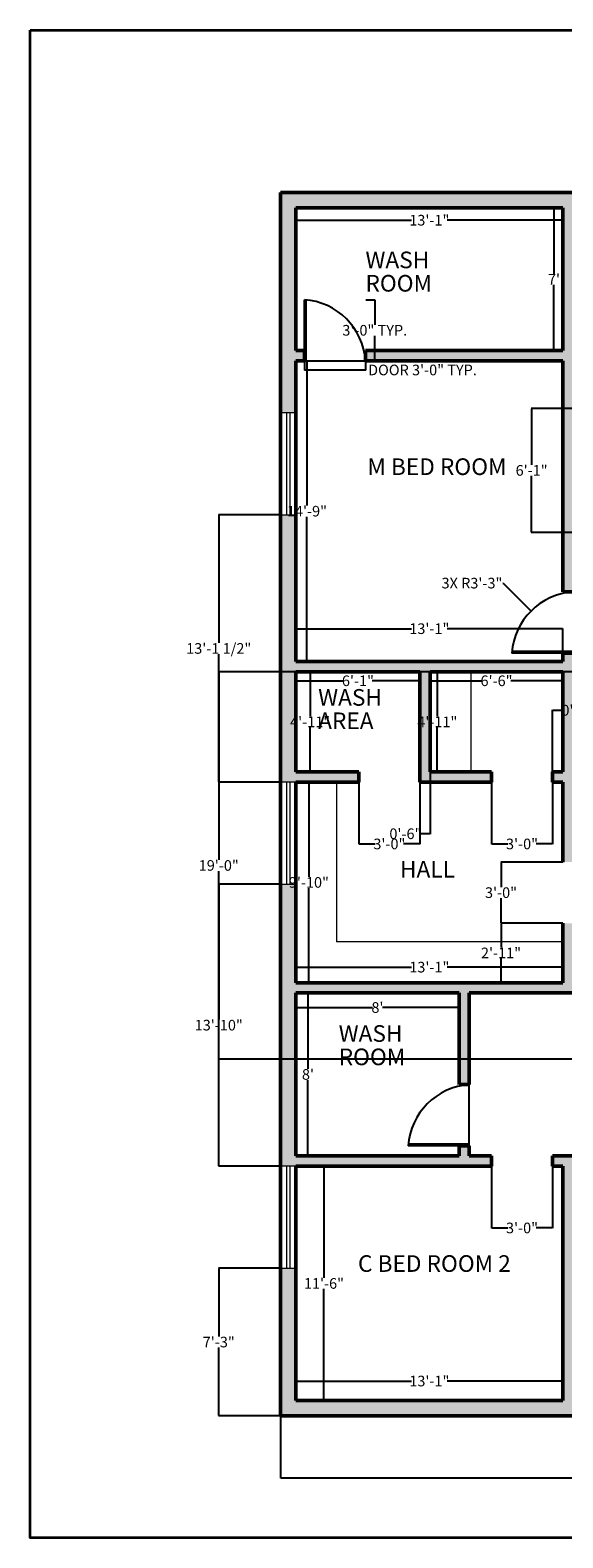
# Model space of a CAD drawing. Units: inches. Extents: x -335 to 1312, y -66 to 821.
# Tile 2 of 4: x 405 to 719, y -66 to 821. Entities that reach past the tile are written whole.
import ezdxf

# ---------------------------------------------------------------- set-up
doc = ezdxf.new("R2010")
doc.units = ezdxf.units.IN
doc.header["$MEASUREMENT"] = 0
for name, color, linetype, lineweight in [('A-ANNO-DIMS', 2, 'Continuous', 18), ('A-ANNO-TTLB', 7, 'Continuous', 35), ('A-AREA-IDEN', 7, 'Continuous', 25), ('A-DOOR', 34, 'Continuous', 25), ('A-FLOR-FIXT', 8, 'Continuous', 18), ('A-GLAZ', 34, 'Continuous', 18), ('A-WALL', 7, 'Continuous', 50), ('A-WALL-PATT', 252, 'Continuous', 13)]:
    doc.layers.add(name, color=color, linetype=linetype, lineweight=lineweight)
doc.styles.get("Standard").update_dxf_attribs({"font": 'arial.ttf'})
doc.dimstyles.get("Standard").update_dxf_attribs({"dimtxt": 6.25, "dimasz": 0.18, "dimexe": 0.18, "dimexo": 0.0625, "dimgap": 0.09, "dimtad": 0, "dimtih": 1, "dimtoh": 1, "dimdec": 0, "dimzin": 0, "dimdsep": 46, "dimlunit": 3, "dimtxsty": 'Standard', "dimcen": 0.09, "dimadec": 0, "dimazin": 0, "dimtfac": 1, "dimtdec": 0, "dimtofl": 0, "dimtmove": 0, "dimatfit": 3, "dimfxl": 1, "dimtolj": 1, "dimtzin": 0, "dimarcsym": 0})

# ---------------------------------------------------------------- blocks, each defined once
blk = doc.blocks.new('*D1')
at = {"layer": 'A-ANNO-DIMS', "color": 0, "lineweight": -2, "transparency": 16777216}
for p, q in [((561.55, 716.35), (561.55, 708.98)), ((718.55, 716.35), (718.55, 708.98)), ((561.73, 709.16), (629.52, 709.16)), ((718.37, 709.16), (650.58, 709.16))]:
    blk.add_line(p, q, dxfattribs=at)
at = {"layer": 'A-ANNO-DIMS', "color": 0, "transparency": 16777216}
for points in [[(561.73, 709.19), (561.73, 709.13), (561.55, 709.16)], [(718.37, 709.19), (718.37, 709.13), (718.55, 709.16)]]:
    blk.add_solid(points, dxfattribs=at)
at = {"layer": 'Defpoints', "color": 0, "transparency": 16777216}
for p in [(561.55, 716.41), (718.55, 716.41), (561.55, 709.16)]:
    blk.add_point(p, dxfattribs=at)
at = {"layer": 'A-ANNO-DIMS', "color": 0, "transparency": 16777216, "insert": (640.05, 709.16), "char_height": 6.25, "attachment_point": 5}
blk.add_mtext('\\A1;13\'-1"', dxfattribs=at)
blk = doc.blocks.new('*D2')
at = {"layer": 'A-ANNO-DIMS', "color": 0, "lineweight": -2, "transparency": 16777216}
for p, q in [((718.49, 716.41), (713.15, 716.41)), ((713.33, 716.23), (713.33, 677.62)), ((713.33, 632.59), (713.33, 671.19)), ((718.49, 632.41), (713.15, 632.41))]:
    blk.add_line(p, q, dxfattribs=at)
at = {"layer": 'A-ANNO-DIMS', "color": 0, "transparency": 16777216}
for points in [[(713.3, 716.23), (713.36, 716.23), (713.33, 716.41)], [(713.3, 632.59), (713.36, 632.59), (713.33, 632.41)]]:
    blk.add_solid(points, dxfattribs=at)
at = {"layer": 'Defpoints', "color": 0, "transparency": 16777216}
for p in [(718.55, 716.41), (713.33, 632.41), (718.55, 632.41)]:
    blk.add_point(p, dxfattribs=at)
at = {"layer": 'A-ANNO-DIMS', "color": 0, "transparency": 16777216, "insert": (713.33, 674.41), "char_height": 6.25, "attachment_point": 5}
blk.add_mtext("\\A1;7'", dxfattribs=at)
blk = doc.blocks.new('*D3')
at = {"layer": 'A-ANNO-DIMS', "color": 0, "lineweight": -2, "transparency": 16777216}
for p, q in [((561.55, 449.47), (561.55, 468.94)), ((561.73, 468.76), (629.52, 468.76)), ((718.37, 468.76), (650.58, 468.76)), ((718.55, 449.47), (718.55, 468.94))]:
    blk.add_line(p, q, dxfattribs=at)
at = {"layer": 'A-ANNO-DIMS', "color": 0, "transparency": 16777216}
for points in [[(561.73, 468.79), (561.73, 468.73), (561.55, 468.76)], [(718.37, 468.79), (718.37, 468.73), (718.55, 468.76)]]:
    blk.add_solid(points, dxfattribs=at)
at = {"layer": 'Defpoints', "color": 0, "transparency": 16777216}
for p in [(561.55, 468.76), (561.55, 449.41), (718.55, 449.41)]:
    blk.add_point(p, dxfattribs=at)
at = {"layer": 'A-ANNO-DIMS', "color": 0, "transparency": 16777216, "insert": (640.05, 468.76), "char_height": 6.25, "attachment_point": 5}
blk.add_mtext('\\A1;13\'-1"', dxfattribs=at)
blk = doc.blocks.new('*D4')
at = {"layer": 'A-ANNO-DIMS', "color": 0, "lineweight": -2, "transparency": 16777216}
for p, q in [((561.61, 626.41), (568.26, 626.41)), ((568.08, 626.23), (568.08, 541.19)), ((568.08, 449.59), (568.08, 534.63)), ((561.61, 449.41), (568.26, 449.41))]:
    blk.add_line(p, q, dxfattribs=at)
at = {"layer": 'A-ANNO-DIMS', "color": 0, "transparency": 16777216}
for points in [[(568.05, 626.23), (568.11, 626.23), (568.08, 626.41)], [(568.05, 449.59), (568.11, 449.59), (568.08, 449.41)]]:
    blk.add_solid(points, dxfattribs=at)
at = {"layer": 'Defpoints', "color": 0, "transparency": 16777216}
for p in [(561.55, 626.41), (561.55, 449.41), (568.08, 449.41)]:
    blk.add_point(p, dxfattribs=at)
at = {"layer": 'A-ANNO-DIMS', "color": 0, "transparency": 16777216, "insert": (568.08, 537.91), "char_height": 6.25, "attachment_point": 5}
blk.add_mtext('\\A1;14\'-9"', dxfattribs=at)
blk = doc.blocks.new('*D5')
at = {"layer": 'A-ANNO-DIMS', "color": 0, "lineweight": -2, "transparency": 16777216}
for p, q in [((561.61, 378.41), (569.39, 378.41)), ((569.21, 378.23), (569.21, 322.69)), ((569.21, 260.59), (569.21, 316.13)), ((561.61, 260.41), (569.39, 260.41))]:
    blk.add_line(p, q, dxfattribs=at)
at = {"layer": 'A-ANNO-DIMS', "color": 0, "transparency": 16777216}
for points in [[(569.18, 378.23), (569.24, 378.23), (569.21, 378.41)], [(569.18, 260.59), (569.24, 260.59), (569.21, 260.41)]]:
    blk.add_solid(points, dxfattribs=at)
at = {"layer": 'Defpoints', "color": 0, "transparency": 16777216}
for p in [(561.55, 378.41), (561.55, 260.41), (569.21, 260.41)]:
    blk.add_point(p, dxfattribs=at)
at = {"layer": 'A-ANNO-DIMS', "color": 0, "transparency": 16777216, "insert": (569.21, 319.41), "char_height": 6.25, "attachment_point": 5}
blk.add_mtext('\\A1;9\'-10"', dxfattribs=at)
blk = doc.blocks.new('*D6')
at = {"layer": 'A-ANNO-DIMS', "color": 0, "lineweight": -2, "transparency": 16777216}
for p, q in [((561.55, 260.47), (561.55, 269.75)), ((561.73, 269.57), (629.52, 269.57)), ((718.37, 269.57), (650.58, 269.57)), ((718.55, 260.47), (718.55, 269.75))]:
    blk.add_line(p, q, dxfattribs=at)
at = {"layer": 'A-ANNO-DIMS', "color": 0, "transparency": 16777216}
for points in [[(561.73, 269.6), (561.73, 269.54), (561.55, 269.57)], [(718.37, 269.6), (718.37, 269.54), (718.55, 269.57)]]:
    blk.add_solid(points, dxfattribs=at)
at = {"layer": 'Defpoints', "color": 0, "transparency": 16777216}
for p in [(561.55, 269.57), (561.55, 260.41), (718.55, 260.41)]:
    blk.add_point(p, dxfattribs=at)
at = {"layer": 'A-ANNO-DIMS', "color": 0, "transparency": 16777216, "insert": (640.05, 269.57), "char_height": 6.25, "attachment_point": 5}
blk.add_mtext('\\A1;13\'-1"', dxfattribs=at)
blk = doc.blocks.new('*D7')
at = {"layer": 'A-ANNO-DIMS', "color": 0, "lineweight": -2, "transparency": 16777216}
for p, q in [((561.55, 443.35), (561.55, 437.91)), ((561.73, 438.09), (589.64, 438.09)), ((634.37, 438.09), (606.47, 438.09)), ((634.55, 443.35), (634.55, 437.91))]:
    blk.add_line(p, q, dxfattribs=at)
at = {"layer": 'A-ANNO-DIMS', "color": 0, "transparency": 16777216}
for points in [[(561.73, 438.12), (561.73, 438.06), (561.55, 438.09)], [(634.37, 438.12), (634.37, 438.06), (634.55, 438.09)]]:
    blk.add_solid(points, dxfattribs=at)
at = {"layer": 'Defpoints', "color": 0, "transparency": 16777216}
for p in [(561.55, 443.41), (561.55, 438.09), (634.55, 443.41)]:
    blk.add_point(p, dxfattribs=at)
at = {"layer": 'A-ANNO-DIMS', "color": 0, "transparency": 16777216, "insert": (598.05, 438.09), "char_height": 6.25, "attachment_point": 5}
blk.add_mtext('\\A1;6\'-1"', dxfattribs=at)
blk = doc.blocks.new('*D8')
at = {"layer": 'A-ANNO-DIMS', "color": 0, "lineweight": -2, "transparency": 16777216}
for p, q in [((561.61, 443.41), (570.12, 443.41)), ((569.94, 443.23), (569.94, 417.14)), ((569.94, 384.59), (569.94, 410.68)), ((561.61, 384.41), (570.12, 384.41))]:
    blk.add_line(p, q, dxfattribs=at)
at = {"layer": 'A-ANNO-DIMS', "color": 0, "transparency": 16777216}
for points in [[(569.91, 443.23), (569.97, 443.23), (569.94, 443.41)], [(569.91, 384.59), (569.97, 384.59), (569.94, 384.41)]]:
    blk.add_solid(points, dxfattribs=at)
at = {"layer": 'Defpoints', "color": 0, "transparency": 16777216}
for p in [(561.55, 443.41), (561.55, 384.41), (569.94, 384.41)]:
    blk.add_point(p, dxfattribs=at)
at = {"layer": 'A-ANNO-DIMS', "color": 0, "transparency": 16777216, "insert": (569.94, 413.91), "char_height": 6.25, "attachment_point": 5}
blk.add_mtext('\\A1;4\'-11"', dxfattribs=at)
blk = doc.blocks.new('*D9')
at = {"layer": 'A-ANNO-DIMS', "color": 0, "lineweight": -2, "transparency": 16777216}
for p, q in [((640.55, 443.35), (640.55, 437.91)), ((640.73, 438.09), (671.14, 438.09)), ((718.37, 438.09), (687.97, 438.09)), ((718.55, 443.35), (718.55, 437.91))]:
    blk.add_line(p, q, dxfattribs=at)
at = {"layer": 'A-ANNO-DIMS', "color": 0, "transparency": 16777216}
for points in [[(640.73, 438.12), (640.73, 438.06), (640.55, 438.09)], [(718.37, 438.12), (718.37, 438.06), (718.55, 438.09)]]:
    blk.add_solid(points, dxfattribs=at)
at = {"layer": 'Defpoints', "color": 0, "transparency": 16777216}
for p in [(640.55, 443.41), (640.55, 438.09), (718.55, 443.41)]:
    blk.add_point(p, dxfattribs=at)
at = {"layer": 'A-ANNO-DIMS', "color": 0, "transparency": 16777216, "insert": (679.55, 438.09), "char_height": 6.25, "attachment_point": 5}
blk.add_mtext('\\A1;6\'-6"', dxfattribs=at)
blk = doc.blocks.new('*D10')
at = {"layer": 'A-ANNO-DIMS', "color": 0, "lineweight": -2, "transparency": 16777216}
for p, q in [((640.61, 443.41), (644.92, 443.41)), ((644.74, 443.23), (644.74, 417.14)), ((644.74, 384.59), (644.74, 410.68)), ((640.61, 384.41), (644.92, 384.41))]:
    blk.add_line(p, q, dxfattribs=at)
at = {"layer": 'A-ANNO-DIMS', "color": 0, "transparency": 16777216}
for points in [[(644.71, 443.23), (644.77, 443.23), (644.74, 443.41)], [(644.71, 384.59), (644.77, 384.59), (644.74, 384.41)]]:
    blk.add_solid(points, dxfattribs=at)
at = {"layer": 'Defpoints', "color": 0, "transparency": 16777216}
for p in [(640.55, 443.41), (640.55, 384.41), (644.74, 384.41)]:
    blk.add_point(p, dxfattribs=at)
at = {"layer": 'A-ANNO-DIMS', "color": 0, "transparency": 16777216, "insert": (644.74, 413.91), "char_height": 6.25, "attachment_point": 5}
blk.add_mtext('\\A1;4\'-11"', dxfattribs=at)
blk = doc.blocks.new('*D11')
at = {"layer": 'A-ANNO-DIMS', "color": 0, "lineweight": -2, "transparency": 16777216}
for p, q in [((561.61, 254.41), (568.85, 254.41)), ((568.67, 254.23), (568.67, 209.69)), ((568.67, 158.59), (568.67, 203.13)), ((561.61, 158.41), (568.85, 158.41))]:
    blk.add_line(p, q, dxfattribs=at)
at = {"layer": 'A-ANNO-DIMS', "color": 0, "transparency": 16777216}
for points in [[(568.64, 254.23), (568.7, 254.23), (568.67, 254.41)], [(568.64, 158.59), (568.7, 158.59), (568.67, 158.41)]]:
    blk.add_solid(points, dxfattribs=at)
at = {"layer": 'Defpoints', "color": 0, "transparency": 16777216}
for p in [(561.55, 254.41), (561.55, 158.41), (568.67, 158.41)]:
    blk.add_point(p, dxfattribs=at)
at = {"layer": 'A-ANNO-DIMS', "color": 0, "transparency": 16777216, "insert": (568.67, 206.41), "char_height": 6.25, "attachment_point": 5}
blk.add_mtext("\\A1;8'", dxfattribs=at)
blk = doc.blocks.new('*D12')
at = {"layer": 'A-ANNO-DIMS', "color": 0, "lineweight": -2, "transparency": 16777216}
for p, q in [((561.55, 254.35), (561.55, 245.62)), ((657.55, 254.35), (657.55, 245.62)), ((561.73, 245.8), (606.58, 245.8)), ((657.37, 245.8), (612.52, 245.8))]:
    blk.add_line(p, q, dxfattribs=at)
at = {"layer": 'A-ANNO-DIMS', "color": 0, "transparency": 16777216}
for points in [[(561.73, 245.83), (561.73, 245.77), (561.55, 245.8)], [(657.37, 245.83), (657.37, 245.77), (657.55, 245.8)]]:
    blk.add_solid(points, dxfattribs=at)
at = {"layer": 'Defpoints', "color": 0, "transparency": 16777216}
for p in [(561.55, 254.41), (657.55, 254.41), (561.55, 245.8)]:
    blk.add_point(p, dxfattribs=at)
at = {"layer": 'A-ANNO-DIMS', "color": 0, "transparency": 16777216, "insert": (609.55, 245.8), "char_height": 6.25, "attachment_point": 5}
blk.add_mtext("\\A1;8'", dxfattribs=at)
blk = doc.blocks.new('*D13')
at = {"layer": 'A-ANNO-DIMS', "color": 0, "lineweight": -2, "transparency": 16777216}
for p, q in [((561.61, 152.41), (578.25, 152.41)), ((578.07, 152.23), (578.07, 86.69)), ((578.07, 14.59), (578.07, 80.13)), ((561.61, 14.41), (578.25, 14.41))]:
    blk.add_line(p, q, dxfattribs=at)
at = {"layer": 'A-ANNO-DIMS', "color": 0, "transparency": 16777216}
for points in [[(578.04, 152.23), (578.1, 152.23), (578.07, 152.41)], [(578.04, 14.59), (578.1, 14.59), (578.07, 14.41)]]:
    blk.add_solid(points, dxfattribs=at)
at = {"layer": 'Defpoints', "color": 0, "transparency": 16777216}
for p in [(561.55, 152.41), (561.55, 14.41), (578.07, 14.41)]:
    blk.add_point(p, dxfattribs=at)
at = {"layer": 'A-ANNO-DIMS', "color": 0, "transparency": 16777216, "insert": (578.07, 83.41), "char_height": 6.25, "attachment_point": 5}
blk.add_mtext('\\A1;11\'-6"', dxfattribs=at)
blk = doc.blocks.new('*D14')
at = {"layer": 'A-ANNO-DIMS', "color": 0, "lineweight": -2, "transparency": 16777216}
for p, q in [((561.55, 14.47), (561.55, 26.14)), ((561.73, 25.96), (629.52, 25.96)), ((718.37, 25.96), (650.58, 25.96)), ((718.55, 14.47), (718.55, 26.14))]:
    blk.add_line(p, q, dxfattribs=at)
at = {"layer": 'A-ANNO-DIMS', "color": 0, "transparency": 16777216}
for points in [[(561.73, 25.99), (561.73, 25.93), (561.55, 25.96)], [(718.37, 25.99), (718.37, 25.93), (718.55, 25.96)]]:
    blk.add_solid(points, dxfattribs=at)
at = {"layer": 'Defpoints', "color": 0, "transparency": 16777216}
for p in [(718.55, 25.96), (561.55, 14.41), (718.55, 14.41)]:
    blk.add_point(p, dxfattribs=at)
at = {"layer": 'A-ANNO-DIMS', "color": 0, "transparency": 16777216, "insert": (640.05, 25.96), "char_height": 6.25, "attachment_point": 5}
blk.add_mtext('\\A1;13\'-1"', dxfattribs=at)
blk = doc.blocks.new('WIN-60IN')
for p, q in [((9, 60), (0, 60)), ((0, 60), (0, 0)), ((3.5, 60), (3.5, 0)), ((5.5, 60), (5.5, 0)), ((9, 0), (9, 60)), ((0, 0), (9, 0))]:
    blk.add_line(p, q)
blk = doc.blocks.new('DOOR-SWING-36IN')
for p, q in [((0, 0), (0, 35.94)), ((1, 0), (1, 35.86)), ((0, 0), (36, 0))]:
    blk.add_line(p, q)
blk.add_arc((-2.68, -2.74), 38.78, 4.05456, 86.03519)
blk = doc.blocks.new('*D27')
at = {"layer": 'A-ANNO-DIMS', "color": 0, "lineweight": -2, "transparency": 16777216}
for p, q in [((566.55, 626.35), (566.55, 620.83)), ((602.55, 626.35), (602.55, 620.83)), ((566.73, 621.01), (602.37, 621.01)), ((602.55, 621.01), (602.73, 621.01))]:
    blk.add_line(p, q, dxfattribs=at)
at = {"layer": 'A-ANNO-DIMS', "color": 0, "transparency": 16777216}
for points in [[(566.73, 621.04), (566.73, 620.98), (566.55, 621.01)], [(602.37, 621.04), (602.37, 620.98), (602.55, 621.01)]]:
    blk.add_solid(points, dxfattribs=at)
at = {"layer": 'Defpoints', "color": 0, "transparency": 16777216}
for p in [(566.55, 626.41), (602.55, 626.41), (602.55, 621.01)]:
    blk.add_point(p, dxfattribs=at)
at = {"layer": 'A-ANNO-DIMS', "color": 0, "transparency": 16777216, "insert": (636.02, 621.01), "char_height": 6.25, "attachment_point": 5}
blk.add_mtext('\\A1;DOOR 3\'-0" TYP.', dxfattribs=at)
blk = doc.blocks.new('*D28')
at = {"layer": 'A-ANNO-DIMS', "color": 0, "lineweight": -2, "transparency": 16777216}
for p, q in [((602.61, 662.35), (608.13, 662.35)), ((607.95, 662.17), (607.95, 647.66)), ((607.95, 626.59), (607.95, 641.1)), ((602.61, 626.41), (608.13, 626.41))]:
    blk.add_line(p, q, dxfattribs=at)
at = {"layer": 'A-ANNO-DIMS', "color": 0, "transparency": 16777216}
for points in [[(607.92, 662.17), (607.98, 662.17), (607.95, 662.35)], [(607.92, 626.59), (607.98, 626.59), (607.95, 626.41)]]:
    blk.add_solid(points, dxfattribs=at)
at = {"layer": 'Defpoints', "color": 0, "transparency": 16777216}
for p in [(602.55, 662.35), (607.95, 662.35), (602.55, 626.41)]:
    blk.add_point(p, dxfattribs=at)
at = {"layer": 'A-ANNO-DIMS', "color": 0, "transparency": 16777216, "insert": (607.95, 644.38), "char_height": 6.25, "attachment_point": 5}
blk.add_mtext('\\A1;3\'-0" TYP.', dxfattribs=at)
blk = doc.blocks.new('*D31')
at = {"layer": 'A-ANNO-DIMS', "color": 0, "lineweight": -2, "transparency": 16777216}
for p, q in [((552.55, 5.35), (552.55, -31.12)), ((1152.55, 5.35), (1152.55, -31.12)), ((552.73, -30.94), (841.73, -30.94)), ((1152.37, -30.94), (863.38, -30.94))]:
    blk.add_line(p, q, dxfattribs=at)
at = {"layer": 'A-ANNO-DIMS', "color": 0, "transparency": 16777216}
for points in [[(552.73, -30.91), (552.73, -30.97), (552.55, -30.94)], [(1152.37, -30.91), (1152.37, -30.97), (1152.55, -30.94)]]:
    blk.add_solid(points, dxfattribs=at)
at = {"layer": 'Defpoints', "color": 0, "transparency": 16777216}
for p in [(552.55, 5.41), (1152.55, 5.41), (1152.55, -30.94)]:
    blk.add_point(p, dxfattribs=at)
at = {"layer": 'A-ANNO-DIMS', "color": 0, "transparency": 16777216, "insert": (852.55, -30.94), "char_height": 6.25, "attachment_point": 5}
blk.add_mtext('\\A1;50\'-0"', dxfattribs=at)
blk = doc.blocks.new('*D33')
at = {"layer": 'A-ANNO-DIMS', "color": 0, "lineweight": -2, "transparency": 16777216}
for p, q in [((1143.49, 443.41), (516.02, 443.41)), ((516.2, 443.23), (516.2, 332.69)), ((516.2, 215.59), (516.2, 326.13)), ((1143.49, 215.41), (516.02, 215.41))]:
    blk.add_line(p, q, dxfattribs=at)
at = {"layer": 'A-ANNO-DIMS', "color": 0, "transparency": 16777216}
for points in [[(516.17, 443.23), (516.23, 443.23), (516.2, 443.41)], [(516.17, 215.59), (516.23, 215.59), (516.2, 215.41)]]:
    blk.add_solid(points, dxfattribs=at)
at = {"layer": 'Defpoints', "color": 0, "transparency": 16777216}
for p in [(516.2, 443.41), (1143.55, 443.41), (1143.55, 215.41)]:
    blk.add_point(p, dxfattribs=at)
at = {"layer": 'A-ANNO-DIMS', "color": 0, "transparency": 16777216, "insert": (516.2, 329.41), "char_height": 6.25, "attachment_point": 5}
blk.add_mtext('\\A1;19\'-0"', dxfattribs=at)
blk = doc.blocks.new('*D34')
at = {"layer": 'A-ANNO-DIMS', "color": 0, "lineweight": -2, "transparency": 16777216}
for p, q in [((736.49, 598.41), (700.02, 598.41)), ((700.2, 598.23), (700.2, 565.19)), ((700.2, 525.59), (700.2, 558.63)), ((736.49, 525.41), (700.02, 525.41))]:
    blk.add_line(p, q, dxfattribs=at)
at = {"layer": 'A-ANNO-DIMS', "color": 0, "transparency": 16777216}
for points in [[(700.17, 598.23), (700.23, 598.23), (700.2, 598.41)], [(700.17, 525.59), (700.23, 525.59), (700.2, 525.41)]]:
    blk.add_solid(points, dxfattribs=at)
at = {"layer": 'Defpoints', "color": 0, "transparency": 16777216}
for p in [(700.2, 598.41), (736.55, 598.41), (736.55, 525.41)]:
    blk.add_point(p, dxfattribs=at)
at = {"layer": 'A-ANNO-DIMS', "color": 0, "transparency": 16777216, "insert": (700.2, 561.91), "char_height": 6.25, "attachment_point": 5}
blk.add_mtext('\\A1;6\'-1"', dxfattribs=at)
blk = doc.blocks.new('*D36')
at = {"layer": 'A-ANNO-DIMS', "color": 0, "lineweight": -2, "transparency": 16777216}
for p, q in [((552.49, 92.41), (516.02, 92.41)), ((516.2, 92.23), (516.2, 52.19)), ((516.2, 5.59), (516.2, 45.63)), ((552.49, 5.41), (516.02, 5.41))]:
    blk.add_line(p, q, dxfattribs=at)
at = {"layer": 'A-ANNO-DIMS', "color": 0, "transparency": 16777216}
for points in [[(516.17, 92.23), (516.23, 92.23), (516.2, 92.41)], [(516.17, 5.59), (516.23, 5.59), (516.2, 5.41)]]:
    blk.add_solid(points, dxfattribs=at)
at = {"layer": 'Defpoints', "color": 0, "transparency": 16777216}
for p in [(516.2, 92.41), (552.55, 92.41), (552.55, 5.41)]:
    blk.add_point(p, dxfattribs=at)
at = {"layer": 'A-ANNO-DIMS', "color": 0, "transparency": 16777216, "insert": (516.2, 48.91), "char_height": 6.25, "attachment_point": 5}
blk.add_mtext('\\A1;7\'-3"', dxfattribs=at)
blk = doc.blocks.new('*D37')
at = {"layer": 'A-ANNO-DIMS', "color": 0, "lineweight": -2, "transparency": 16777216}
for p, q in [((552.49, 318.41), (516.02, 318.41)), ((516.2, 318.23), (516.2, 238.69)), ((516.2, 152.59), (516.2, 232.13)), ((552.49, 152.41), (516.02, 152.41))]:
    blk.add_line(p, q, dxfattribs=at)
at = {"layer": 'A-ANNO-DIMS', "color": 0, "transparency": 16777216}
for points in [[(516.17, 318.23), (516.23, 318.23), (516.2, 318.41)], [(516.17, 152.59), (516.23, 152.59), (516.2, 152.41)]]:
    blk.add_solid(points, dxfattribs=at)
at = {"layer": 'Defpoints', "color": 0, "transparency": 16777216}
for p in [(516.2, 318.41), (552.55, 318.41), (552.55, 152.41)]:
    blk.add_point(p, dxfattribs=at)
at = {"layer": 'A-ANNO-DIMS', "color": 0, "transparency": 16777216, "insert": (516.2, 235.41), "char_height": 6.25, "attachment_point": 5}
blk.add_mtext('\\A1;13\'-10"', dxfattribs=at)
blk = doc.blocks.new('*D38')
at = {"layer": 'A-ANNO-DIMS', "color": 0, "lineweight": -2, "transparency": 16777216}
for p, q in [((552.49, 535.84), (516.02, 535.84)), ((516.2, 535.66), (516.2, 460.45)), ((516.2, 378.59), (516.2, 453.8)), ((552.49, 378.41), (516.02, 378.41))]:
    blk.add_line(p, q, dxfattribs=at)
at = {"layer": 'A-ANNO-DIMS', "color": 0, "transparency": 16777216}
for points in [[(516.17, 535.66), (516.23, 535.66), (516.2, 535.84)], [(516.17, 378.59), (516.23, 378.59), (516.2, 378.41)]]:
    blk.add_solid(points, dxfattribs=at)
at = {"layer": 'Defpoints', "color": 0, "transparency": 16777216}
for p in [(516.2, 535.84), (552.55, 535.84), (552.55, 378.41)]:
    blk.add_point(p, dxfattribs=at)
at = {"layer": 'A-ANNO-DIMS', "color": 0, "transparency": 16777216, "insert": (516.2, 457.12), "char_height": 6.25, "attachment_point": 5}
blk.add_mtext('\\A1;13\'-1 1/2"', dxfattribs=at)
blk = doc.blocks.new('*D53')
at = {"layer": 'A-ANNO-DIMS', "color": 0, "lineweight": -2, "transparency": 16777216}
for p, q in [((598.55, 378.35), (598.55, 341.88)), ((634.55, 378.35), (634.55, 341.88)), ((598.73, 342.06), (608.16, 342.06)), ((634.37, 342.06), (624.95, 342.06))]:
    blk.add_line(p, q, dxfattribs=at)
at = {"layer": 'A-ANNO-DIMS', "color": 0, "transparency": 16777216}
for points in [[(598.73, 342.09), (598.73, 342.03), (598.55, 342.06)], [(634.37, 342.09), (634.37, 342.03), (634.55, 342.06)]]:
    blk.add_solid(points, dxfattribs=at)
at = {"layer": 'Defpoints', "color": 0, "transparency": 16777216}
for p in [(598.55, 378.41), (634.55, 378.41), (598.55, 342.06)]:
    blk.add_point(p, dxfattribs=at)
at = {"layer": 'A-ANNO-DIMS', "color": 0, "transparency": 16777216, "insert": (616.55, 342.06), "char_height": 6.25, "attachment_point": 5}
blk.add_mtext('\\A1;3\'-0"', dxfattribs=at)
blk = doc.blocks.new('*D54')
at = {"layer": 'A-ANNO-DIMS', "color": 0, "lineweight": -2, "transparency": 16777216}
for p, q in [((676.55, 378.35), (676.55, 341.88)), ((712.55, 378.35), (712.55, 341.88)), ((676.73, 342.06), (686.16, 342.06)), ((712.37, 342.06), (702.95, 342.06))]:
    blk.add_line(p, q, dxfattribs=at)
at = {"layer": 'A-ANNO-DIMS', "color": 0, "transparency": 16777216}
for points in [[(676.73, 342.09), (676.73, 342.03), (676.55, 342.06)], [(712.37, 342.09), (712.37, 342.03), (712.55, 342.06)]]:
    blk.add_solid(points, dxfattribs=at)
at = {"layer": 'Defpoints', "color": 0, "transparency": 16777216}
for p in [(676.55, 378.41), (712.55, 378.41), (676.55, 342.06)]:
    blk.add_point(p, dxfattribs=at)
at = {"layer": 'A-ANNO-DIMS', "color": 0, "transparency": 16777216, "insert": (694.55, 342.06), "char_height": 6.25, "attachment_point": 5}
blk.add_mtext('\\A1;3\'-0"', dxfattribs=at)
blk = doc.blocks.new('*D55')
at = {"layer": 'A-ANNO-DIMS', "color": 0, "lineweight": -2, "transparency": 16777216}
for p, q in [((718.49, 331.41), (682.02, 331.41)), ((682.2, 331.23), (682.2, 316.69)), ((682.2, 295.59), (682.2, 310.13)), ((718.49, 295.41), (682.02, 295.41))]:
    blk.add_line(p, q, dxfattribs=at)
at = {"layer": 'A-ANNO-DIMS', "color": 0, "transparency": 16777216}
for points in [[(682.17, 331.23), (682.23, 331.23), (682.2, 331.41)], [(682.17, 295.59), (682.23, 295.59), (682.2, 295.41)]]:
    blk.add_solid(points, dxfattribs=at)
at = {"layer": 'Defpoints', "color": 0, "transparency": 16777216}
for p in [(682.2, 331.41), (718.55, 331.41), (718.55, 295.41)]:
    blk.add_point(p, dxfattribs=at)
at = {"layer": 'A-ANNO-DIMS', "color": 0, "transparency": 16777216, "insert": (682.2, 313.41), "char_height": 6.25, "attachment_point": 5}
blk.add_mtext('\\A1;3\'-0"', dxfattribs=at)
blk = doc.blocks.new('*D56')
at = {"layer": 'A-ANNO-DIMS', "color": 0, "lineweight": -2, "transparency": 16777216}
for p, q in [((676.55, 152.35), (676.55, 115.88)), ((712.55, 152.35), (712.55, 115.88)), ((676.73, 116.06), (686.16, 116.06)), ((712.37, 116.06), (702.95, 116.06))]:
    blk.add_line(p, q, dxfattribs=at)
at = {"layer": 'A-ANNO-DIMS', "color": 0, "transparency": 16777216}
for points in [[(676.73, 116.09), (676.73, 116.03), (676.55, 116.06)], [(712.37, 116.09), (712.37, 116.03), (712.55, 116.06)]]:
    blk.add_solid(points, dxfattribs=at)
at = {"layer": 'Defpoints', "color": 0, "transparency": 16777216}
for p in [(676.55, 152.41), (712.55, 152.41), (676.55, 116.06)]:
    blk.add_point(p, dxfattribs=at)
at = {"layer": 'A-ANNO-DIMS', "color": 0, "transparency": 16777216, "insert": (694.55, 116.06), "char_height": 6.25, "attachment_point": 5}
blk.add_mtext('\\A1;3\'-0"', dxfattribs=at)
blk = doc.blocks.new('*D59')
at = {"layer": 'A-ANNO-DIMS', "color": 0, "lineweight": -2, "transparency": 16777216}
for p, q in [((634.55, 384.35), (634.55, 347.88)), ((640.55, 384.35), (640.55, 347.88)), ((634.55, 348.06), (634.37, 348.06)), ((640.37, 348.06), (634.73, 348.06))]:
    blk.add_line(p, q, dxfattribs=at)
at = {"layer": 'A-ANNO-DIMS', "color": 0, "transparency": 16777216}
for points in [[(634.73, 348.09), (634.73, 348.03), (634.55, 348.06)], [(640.37, 348.09), (640.37, 348.03), (640.55, 348.06)]]:
    blk.add_solid(points, dxfattribs=at)
at = {"layer": 'Defpoints', "color": 0, "transparency": 16777216}
for p in [(634.55, 384.41), (640.55, 384.41), (634.55, 348.06)]:
    blk.add_point(p, dxfattribs=at)
at = {"layer": 'A-ANNO-DIMS', "color": 0, "transparency": 16777216, "insert": (625.97, 348.06), "char_height": 6.25, "attachment_point": 5}
blk.add_mtext('\\A1;0\'-6"', dxfattribs=at)
blk = doc.blocks.new('*D60')
at = {"layer": 'A-ANNO-DIMS', "color": 0, "lineweight": -2, "transparency": 16777216}
for p, q in [((718.49, 295.41), (682.02, 295.41)), ((682.2, 295.23), (682.2, 281.14)), ((682.2, 260.59), (682.2, 274.68)), ((718.49, 260.41), (682.02, 260.41))]:
    blk.add_line(p, q, dxfattribs=at)
at = {"layer": 'A-ANNO-DIMS', "color": 0, "transparency": 16777216}
for points in [[(682.17, 295.23), (682.23, 295.23), (682.2, 295.41)], [(682.17, 260.59), (682.23, 260.59), (682.2, 260.41)]]:
    blk.add_solid(points, dxfattribs=at)
at = {"layer": 'Defpoints', "color": 0, "transparency": 16777216}
for p in [(682.2, 295.41), (718.55, 295.41), (718.55, 260.41)]:
    blk.add_point(p, dxfattribs=at)
at = {"layer": 'A-ANNO-DIMS', "color": 0, "transparency": 16777216, "insert": (682.2, 277.91), "char_height": 6.25, "attachment_point": 5}
blk.add_mtext('\\A1;2\'-11"', dxfattribs=at)
blk = doc.blocks.new('*D61')
at = {"layer": 'A-ANNO-DIMS', "color": 0, "lineweight": -2, "transparency": 16777216}
for p, q in [((712.55, 384.47), (712.55, 420.94)), ((712.73, 420.76), (718.37, 420.76)), ((718.55, 384.47), (718.55, 420.94)), ((718.55, 420.76), (718.73, 420.76))]:
    blk.add_line(p, q, dxfattribs=at)
at = {"layer": 'A-ANNO-DIMS', "color": 0, "transparency": 16777216}
for points in [[(712.73, 420.79), (712.73, 420.73), (712.55, 420.76)], [(718.37, 420.79), (718.37, 420.73), (718.55, 420.76)]]:
    blk.add_solid(points, dxfattribs=at)
at = {"layer": 'Defpoints', "color": 0, "transparency": 16777216}
for p in [(718.55, 420.76), (712.55, 384.41), (718.55, 384.41)]:
    blk.add_point(p, dxfattribs=at)
at = {"layer": 'A-ANNO-DIMS', "color": 0, "transparency": 16777216, "insert": (727.13, 420.76), "char_height": 6.25, "attachment_point": 5}
blk.add_mtext('\\A1;0\'-6"', dxfattribs=at)
blk = doc.blocks.new('*D62')
at = {"layer": 'A-ANNO-DIMS', "color": 0, "lineweight": -2, "transparency": 16777216}
for p, q in [((683.21, 495.57), (683.39, 495.57)), ((683.39, 495.57), (699.72, 479.25)), ((727.2, 451.73), (727.38, 451.73)), ((727.29, 451.64), (727.29, 451.82))]:
    blk.add_line(p, q, dxfattribs=at)
at = {"layer": 'A-ANNO-DIMS', "color": 0, "transparency": 16777216}
blk.add_solid([(699.74, 479.27), (699.7, 479.23), (699.85, 479.13)], dxfattribs=at)
at = {"layer": 'Defpoints', "color": 0, "transparency": 16777216}
for p in [(699.85, 479.13), (727.29, 451.73)]:
    blk.add_point(p, dxfattribs=at)
at = {"layer": 'A-ANNO-DIMS', "color": 0, "transparency": 16777216, "insert": (665.11, 495.57), "char_height": 6.25, "attachment_point": 5}
blk.add_mtext('\\A1;3X R3\'-3"', dxfattribs=at)

msp = doc.modelspace()

# ---------------------------------------------------------------- hatches: boundary and pattern name
at = {"layer": 'A-WALL-PATT'}
h = msp.add_hatch(color=256, dxfattribs=at)
h.dxf.hatch_style = 1
h.paths.add_polyline_path([(561.55, 92.41), (552.55, 92.41), (552.55, 5.41), (724.55, 5.41), (724.55, 84.41), (727.55, 84.41), (727.55, 93.41), (724.55, 93.41), (724.55, 158.41), (712.55, 158.41), (712.55, 152.41), (718.55, 152.41), (718.55, 14.41), (561.55, 14.41)])
h.paths.add_polyline_path([(561.55, 254.41), (657.55, 254.41), (657.55, 200.41), (663.55, 200.41), (663.55, 254.41), (724.55, 254.41), (724.55, 278.41), (728.55, 278.41), (728.55, 283.41), (724.55, 283.41), (724.55, 295.41), (718.55, 295.41), (718.55, 260.41), (561.55, 260.41), (561.55, 318.41), (552.55, 318.41), (552.55, 152.41), (561.55, 152.41), (676.55, 152.41), (676.55, 158.41), (663.55, 158.41), (663.55, 164.41), (657.55, 164.41), (657.55, 158.41), (561.55, 158.41)])
h.paths.add_polyline_path([(561.55, 443.41), (634.55, 443.41), (634.55, 384.41), (634.55, 378.41), (676.55, 378.41), (676.55, 384.41), (640.55, 384.41), (640.55, 443.41), (718.55, 443.41), (718.55, 384.41), (712.55, 384.41), (712.55, 378.41), (718.55, 378.41), (718.55, 331.41), (724.55, 331.41), (724.55, 454.41), (718.55, 454.41), (718.55, 449.41), (561.55, 449.41), (561.55, 535.84), (552.55, 535.84), (552.55, 378.41), (561.55, 378.41), (598.55, 378.41), (598.55, 384.41), (561.55, 384.41)])
h.paths.add_polyline_path([(724.55, 725.41), (552.55, 725.41), (552.55, 595.84), (561.55, 595.84), (561.55, 626.41), (566.55, 626.41), (566.55, 632.41), (561.55, 632.41), (561.55, 716.41), (718.55, 716.41), (718.55, 632.41), (602.55, 632.41), (602.55, 626.41), (718.55, 626.41), (718.55, 490.41), (724.55, 490.41), (724.55, 519.41), (772.54, 519.41), (772.56, 525.41), (724.55, 525.41)])
h.paths.add_polyline_path([(927.55, 716.41), (1143.55, 716.41), (1143.55, 632.41), (1139.31, 632.41), (1139.31, 626.41), (1143.55, 626.41), (1143.55, 598.07), (1152.55, 598.07), (1152.55, 725.41), (921.55, 725.41), (921.55, 598.41), (921.55, 525.41), (904.55, 525.41), (904.55, 519.41), (921.55, 519.41), (921.55, 490.41), (927.55, 490.41), (927.55, 626.41), (1103.31, 626.41), (1103.31, 632.41), (927.55, 632.41)])
h.paths.add_polyline_path([(1152.55, 538.07), (1143.55, 538.07), (1143.55, 449.41), (927.55, 449.41), (927.55, 454.41), (921.55, 454.41), (921.55, 283.41), (764.57, 283.41), (764.55, 278.41), (921.55, 278.41), (921.55, 261.75), (927.55, 261.75), (927.55, 443.41), (1143.55, 443.41), (1143.55, 284.87), (1152.55, 284.87)])
h.paths.add_polyline_path([(930.55, 206.41), (1143.55, 206.41), (1143.55, 215.41), (927.55, 215.41), (927.55, 225.75), (921.55, 225.75), (921.55, 93.41), (857.84, 93.41), (857.84, 84.41), (930.55, 84.41)])
h.paths.add_polyline_path([(1152.55, 206.41), (1143.55, 206.41), (1143.55, 5.41), (1152.55, 5.41)])
h.paths.add_polyline_path([(797.84, 93.41), (763.55, 93.41), (763.55, 84.41), (797.84, 84.41)])

# ---------------------------------------------------------------- linework, layer by layer
at = {"layer": 'A-ANNO-TTLB'}
msp.add_lwpolyline([(405.31, 821.01), (1312, 821.01), (1312, -66.33), (405.31, -66.33)], close=True, dxfattribs=at)
at = {"layer": 'A-FLOR-FIXT'}
for p, q in [((664.55, 443.41), (664.55, 384.41)), ((585.55, 378.41), (585.55, 284.41)), ((718.55, 284.41), (585.55, 284.41))]:
    msp.add_line(p, q, dxfattribs=at)
at = {"layer": 'A-WALL'}
for p, q in [((1152.55, 725.41), (552.55, 725.41)), ((552.55, 725.41), (552.55, 5.41)), ((561.55, 716.41), (561.55, 632.41)), ((718.55, 716.41), (561.55, 716.41)), ((718.55, 716.41), (718.55, 632.41)), ((566.55, 632.41), (561.55, 632.41)), ((566.55, 632.41), (566.55, 626.41)), ((718.55, 632.41), (602.55, 632.41)), ((602.55, 632.41), (602.55, 626.41)), ((561.55, 626.41), (561.55, 449.41)), ((566.55, 626.41), (561.55, 626.41)), ((718.55, 626.41), (602.55, 626.41)), ((718.55, 626.41), (718.55, 490.41)), ((718.55, 490.41), (724.55, 490.41)), ((718.55, 454.41), (724.55, 454.41)), ((718.55, 454.41), (718.55, 449.41)), ((718.55, 449.41), (561.55, 449.41)), ((561.55, 443.41), (561.55, 384.41)), ((634.55, 443.41), (561.55, 443.41)), ((634.55, 443.41), (634.55, 384.41)), ((718.55, 443.41), (640.55, 443.41)), ((640.55, 443.41), (640.55, 384.41)), ((718.55, 443.41), (718.55, 384.41)), ((598.55, 384.41), (561.55, 384.41)), ((598.55, 384.41), (598.55, 378.41)), ((634.55, 384.41), (634.55, 378.41)), ((676.55, 384.41), (640.55, 384.41)), ((676.55, 378.41), (676.55, 384.41)), ((718.55, 384.41), (712.55, 384.41)), ((712.55, 378.41), (712.55, 384.41)), ((561.55, 378.41), (561.55, 260.41)), ((598.55, 378.41), (561.55, 378.41)), ((676.55, 378.41), (634.55, 378.41)), ((718.55, 378.41), (712.55, 378.41)), ((718.55, 378.41), (718.55, 331.41)), ((718.55, 295.41), (718.55, 260.41)), ((718.55, 260.41), (561.55, 260.41)), ((561.55, 254.41), (561.55, 158.41)), ((657.55, 254.41), (561.55, 254.41)), ((657.55, 254.41), (657.55, 200.41)), ((724.55, 254.41), (663.55, 254.41)), ((663.55, 254.41), (663.55, 200.41)), ((657.55, 200.41), (663.55, 200.41)), ((657.55, 164.41), (663.55, 164.41)), ((657.55, 164.41), (657.55, 158.41)), ((663.55, 164.41), (663.55, 158.41)), ((561.55, 158.41), (657.55, 158.41)), ((561.55, 152.41), (676.55, 152.41)), ((561.55, 152.41), (561.55, 14.41)), ((663.55, 158.41), (676.55, 158.41)), ((676.55, 152.41), (676.55, 158.41)), ((712.55, 152.41), (712.55, 158.41)), ((712.55, 158.41), (724.55, 158.41)), ((712.55, 152.41), (718.55, 152.41)), ((718.55, 152.41), (718.55, 14.41)), ((561.55, 14.41), (718.55, 14.41)), ((552.55, 5.41), (724.55, 5.41))]:
    msp.add_line(p, q, dxfattribs=at)

# ---------------------------------------------------------------- block references
at = {"layer": 'A-DOOR'}
msp.add_blockref('DOOR-SWING-36IN', (566.55, 626.41), dxfattribs=at)
for p, rotation in [((724.55, 454.41), 89.99999999999935), ((663.55, 164.41), 89.99999999999928)]:
    msp.add_blockref('DOOR-SWING-36IN', p, dxfattribs=dict(at, rotation=rotation))
at = {"layer": 'A-GLAZ'}
for p in [(552.55, 535.84), (552.55, 318.41), (552.55, 92.41)]:
    msp.add_blockref('WIN-60IN', p, dxfattribs=at)

# ---------------------------------------------------------------- texts
at = {"layer": 'A-AREA-IDEN'}
for s, height, p in [('WASH ', 9.789, (602.48, 680.9)), ('ROOM', 9.789, (602.48, 667.15)), ('M BED ROOM', 9.789, (603.62, 559.2)), ('WASH ', 9.789, (574.67, 423.41)), ('AREA', 9.789, (574.67, 409.65)), ('HALL', 9.789, (622.79, 322.31)), ('WASH ', 9.789, (586.73, 225.6)), ('ROOM', 9.789, (586.73, 211.85)), ('C BED ROOM 2', 9.7886, (598.09, 90.22))]:
    msp.add_text(s, height=height, dxfattribs=at).set_placement(p)

# ---------------------------------------------------------------- dimensions: what is measured, and where the dimension line sits
at = {"layer": 'A-ANNO-DIMS'}
for base, p1, p2, override, picture, middle in [((561.55, 709.16), (718.55, 716.41), (561.55, 716.41), {"dimclrd": 0, "dimclre": 0, "dimclrt": 0}, '*D1', (640.05, 709.16)), ((561.55, 468.76), (718.55, 449.41), (561.55, 449.41), {"dimclrd": 0, "dimclre": 0, "dimclrt": 0}, '*D3', (640.05, 468.76)), ((561.55, 438.09), (634.55, 443.41), (561.55, 443.41), {"dimclrd": 0, "dimclre": 0, "dimclrt": 0}, '*D7', (598.05, 438.09)), ((640.55, 438.09), (718.55, 443.41), (640.55, 443.41), {"dimclrd": 0, "dimclre": 0, "dimclrt": 0}, '*D9', (679.55, 438.09)), ((718.55, 420.76), (712.55, 384.41), (718.55, 384.41), {"dimdec": 1, "dimlfac": 1, "dimrnd": 0, "dimzin": 1, "dimdsep": 46, "dimlunit": 4, "dimfrac": 2}, '*D61', (727.13, 420.76)), ((561.55, 269.57), (718.55, 260.41), (561.55, 260.41), {"dimclrd": 0, "dimclre": 0, "dimclrt": 0}, '*D6', (640.05, 269.57)), ((561.55, 245.8), (657.55, 254.41), (561.55, 254.41), {"dimclrd": 0, "dimclre": 0, "dimclrt": 0}, '*D12', (609.55, 245.8)), ((718.55, 25.96), (561.55, 14.41), (718.55, 14.41), {"dimclrd": 0, "dimclre": 0, "dimclrt": 0}, '*D14', (640.05, 25.96)), ((1152.55, -30.94), (552.55, 5.41), (1152.55, 5.41), {"dimdec": 1, "dimlfac": 1, "dimrnd": 0, "dimzin": 1, "dimdsep": 46, "dimlunit": 4, "dimfrac": 2}, '*D31', (852.55, -30.94))]:
    dim = msp.add_linear_dim(base=base, p1=p1, p2=p2, dimstyle='Standard', override=override, dxfattribs=at)
    dim.commit()
    dim.dimension.update_dxf_attribs({"geometry": picture, "text_midpoint": middle})
for base, p1, p2, angle, override, picture, middle in [((713.33, 632.41), (718.55, 716.41), (718.55, 632.41), 90, {"dimclrd": 0, "dimclre": 0, "dimclrt": 0}, '*D2', (713.33, 674.41)), ((568.08, 449.41), (561.55, 626.41), (561.55, 449.41), 90, {"dimclrd": 0, "dimclre": 0, "dimclrt": 0}, '*D4', (568.08, 537.91)), ((700.2, 598.41), (736.55, 525.41), (736.55, 598.41), 90, {"dimdec": 1, "dimlfac": 1, "dimrnd": 0, "dimzin": 1, "dimdsep": 46, "dimlunit": 4, "dimfrac": 2}, '*D34', (700.2, 561.91)), ((516.2, 535.84), (552.55, 378.41), (552.55, 535.84), 90, {"dimdec": 1, "dimlfac": 1, "dimrnd": 0, "dimzin": 1, "dimdsep": 46, "dimlunit": 4, "dimfrac": 2}, '*D38', (516.2, 457.12)), ((516.2, 443.41), (1143.55, 215.41), (1143.55, 443.41), 90, {"dimdec": 1, "dimlfac": 1, "dimrnd": 0, "dimzin": 1, "dimdsep": 46, "dimlunit": 4, "dimfrac": 2}, '*D33', (516.2, 329.41)), ((569.94, 384.41), (561.55, 443.41), (561.55, 384.41), 90, {"dimclrd": 0, "dimclre": 0, "dimclrt": 0}, '*D8', (569.94, 413.91)), ((644.74, 384.41), (640.55, 443.41), (640.55, 384.41), 90, {"dimclrd": 0, "dimclre": 0, "dimclrt": 0}, '*D10', (644.74, 413.91)), ((634.55, 348.06), (640.55, 384.41), (634.55, 384.41), 180, {"dimdec": 1, "dimlfac": 1, "dimrnd": 0, "dimzin": 1, "dimdsep": 46, "dimlunit": 4, "dimfrac": 2}, '*D59', (625.97, 348.06)), ((569.21, 260.41), (561.55, 378.41), (561.55, 260.41), 90, {"dimclrd": 0, "dimclre": 0, "dimclrt": 0}, '*D5', (569.21, 319.41)), ((598.55, 342.06), (634.55, 378.41), (598.55, 378.41), 180, {"dimdec": 1, "dimlfac": 1, "dimrnd": 0, "dimzin": 1, "dimdsep": 46, "dimlunit": 4, "dimfrac": 2}, '*D53', (616.55, 342.06)), ((676.55, 342.06), (712.55, 378.41), (676.55, 378.41), 180, {"dimdec": 1, "dimlfac": 1, "dimrnd": 0, "dimzin": 1, "dimdsep": 46, "dimlunit": 4, "dimfrac": 2}, '*D54', (694.55, 342.06)), ((682.2, 331.41), (718.55, 295.41), (718.55, 331.41), 90, {"dimdec": 1, "dimlfac": 1, "dimrnd": 0, "dimzin": 1, "dimdsep": 46, "dimlunit": 4, "dimfrac": 2}, '*D55', (682.2, 313.41)), ((516.2, 318.41), (552.55, 152.41), (552.55, 318.41), 90, {"dimdec": 1, "dimlfac": 1, "dimrnd": 0, "dimzin": 1, "dimdsep": 46, "dimlunit": 4, "dimfrac": 2}, '*D37', (516.2, 235.41)), ((682.2, 295.41), (718.55, 260.41), (718.55, 295.41), 90, {"dimdec": 1, "dimlfac": 1, "dimrnd": 0, "dimzin": 1, "dimdsep": 46, "dimlunit": 4, "dimfrac": 2}, '*D60', (682.2, 277.91)), ((568.67, 158.41), (561.55, 254.41), (561.55, 158.41), 90, {"dimclrd": 0, "dimclre": 0, "dimclrt": 0}, '*D11', (568.67, 206.41)), ((578.07, 14.41), (561.55, 152.41), (561.55, 14.41), 90, {"dimclrd": 0, "dimclre": 0, "dimclrt": 0}, '*D13', (578.07, 83.41)), ((676.55, 116.06), (712.55, 152.41), (676.55, 152.41), 180, {"dimdec": 1, "dimlfac": 1, "dimrnd": 0, "dimzin": 1, "dimdsep": 46, "dimlunit": 4, "dimfrac": 2}, '*D56', (694.55, 116.06)), ((516.2, 92.41), (552.55, 5.41), (552.55, 92.41), 90, {"dimdec": 1, "dimlfac": 1, "dimrnd": 0, "dimzin": 1, "dimdsep": 46, "dimlunit": 4, "dimfrac": 2}, '*D36', (516.2, 48.91))]:
    dim = msp.add_linear_dim(base=base, p1=p1, p2=p2, angle=angle, dimstyle='Standard', override=override, dxfattribs=at)
    dim.commit()
    dim.dimension.update_dxf_attribs({"geometry": picture, "text_midpoint": middle})
dim = msp.add_linear_dim(base=(607.95, 662.35), p1=(602.55, 626.41), p2=(602.55, 662.35), angle=90, text='<> TYP.', dimstyle='Standard', override={"dimdec": 1, "dimlfac": 1, "dimrnd": 0, "dimzin": 1, "dimdsep": 46, "dimlunit": 4, "dimfrac": 2}, dxfattribs=at)
dim.commit()
dim.dimension.update_dxf_attribs({"geometry": '*D28', "text_midpoint": (607.95, 644.38)})
dim = msp.add_linear_dim(base=(602.55, 621.01), p1=(566.55, 626.41), p2=(602.55, 626.41), text='DOOR <> TYP.', dimstyle='Standard', override={"dimdec": 1, "dimlfac": 1, "dimrnd": 0, "dimzin": 1, "dimdsep": 46, "dimlunit": 4, "dimfrac": 2}, dxfattribs=at)
dim.commit()
dim.dimension.update_dxf_attribs({"geometry": '*D27', "text_midpoint": (636.02, 621.01)})
dim = msp.add_radius_dim(center=(727.29, 451.73), mpoint=(699.85, 479.13), text='3X <>', dimstyle='Standard', override={"dimdec": 1, "dimlfac": 1, "dimrnd": 0, "dimzin": 1, "dimdsep": 46, "dimlunit": 4, "dimfrac": 2}, dxfattribs=at)
dim.commit()
dim.dimension.update_dxf_attribs({"geometry": '*D62', "text_midpoint": (665.11, 495.57), "dimtype": 164})

doc.saveas('drawing.dxf')
